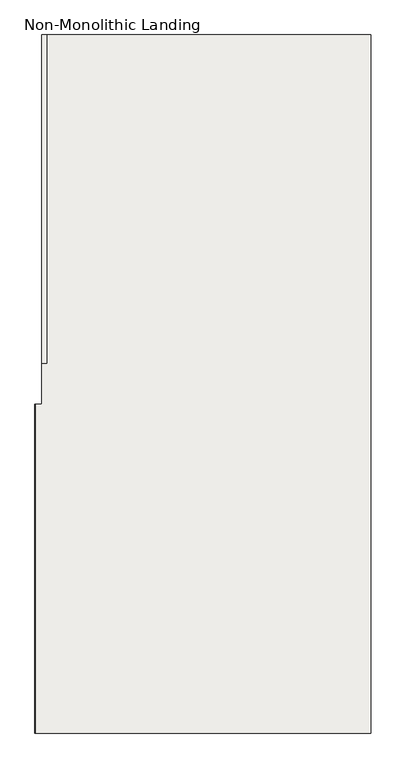
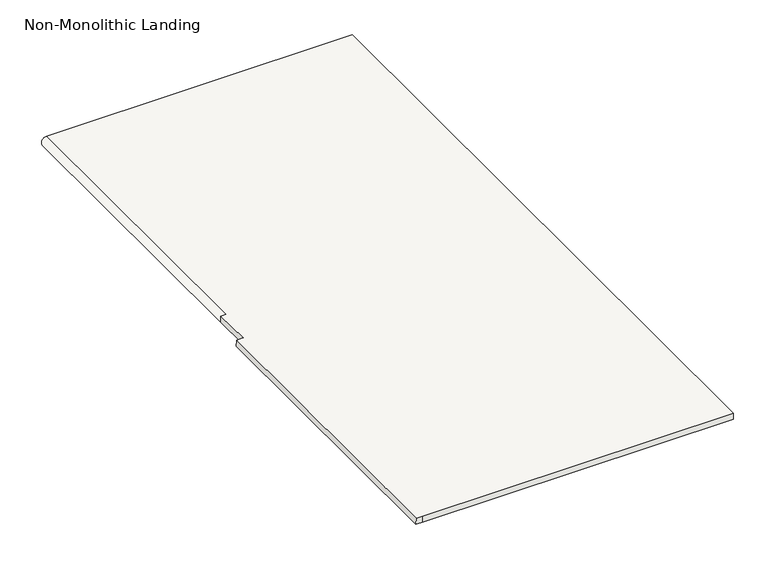
"""IFC4 building model written with IfcOpenShell, lengths in millimetres: slab geometry, Non-Monolithic Landing."""

from ifc_helpers import new_model, si_unit, frame, origin, place, context, project, spatial, circle_curve, source, transform, mapped, element, save
from ifc_brep_helpers import plane_surface, cylinder_surface, advanced_brep


def non_monolithic_landing_c74da7f8(model_context):
    return source(origin(), model_context, "Body", "AdvancedBrep", [
        advanced_brep(
        [(9872.4583908, 2257.2640673, 1676.4), (9871.3284975, 2257.2640673, 1651.0), (9871.3284975, 1038.0640673, 1651.0), (9872.4583908, 1038.0640673, 1676.4), (9917.4583908, 2407.2640673, 1676.4), (9897.4583908, 2407.2640673, 1676.4), (9897.4583908, 2257.2640673, 1676.4), (9897.4583908, 1038.0640673, 1676.4), (11116.6583908, 1038.0640673, 1676.4), (11116.6583908, 3626.4640673, 1676.4), (9917.4583908, 3626.4640673, 1676.4), (9897.4583908, 2257.2640673, 1651.0), (9897.4583908, 2407.2640673, 1651.0), (9898.2011843, 2407.2640673, 1651.0), (9917.4583908, 2407.2640673, 1651.0), (9917.4583908, 3626.4640673, 1651.0), (11116.6583908, 3626.4640673, 1651.0), (11116.6583908, 1038.0640673, 1651.0), (9897.4583908, 1038.0640673, 1651.0), (9897.4583908, 2407.2640673, 1656.4), (9917.4583908, 3626.4640673, 1636.4), (9917.4583908, 2407.2640673, 1636.4)],
        [
            (0, 1),
            (1, 2),
            (2, 3),
            (3, 0),
            (4, 5),
            (5, 6),
            (6, 0),
            (3, 7),
            (7, 8),
            (8, 9),
            (9, 10),
            (10, 4),
            (11, 12),
            (12, 13),
            (13, 14),
            (14, 15),
            (15, 16),
            (16, 17),
            (17, 18),
            (18, 2),
            (1, 11),
            (4, 19, circle_curve(frame((9917.4583908, 2407.2640673, 1656.4), z_axis=(0.0, -1.0, 0.0), x_axis=(1.0, 0.0, 0.0)), 20.0)),
            (19, 5),
            (12, 19),
            (19, 13, circle_curve(frame((9917.4583908, 2407.2640673, 1656.4), z_axis=(0.0, -1.0, 0.0), x_axis=(1.0, 0.0, 0.0)), 20.0)),
            (11, 6),
            (18, 7),
            (17, 8),
            (16, 9),
            (15, 20),
            (20, 10, circle_curve(frame((9917.4583908, 3626.4640673, 1656.4), z_axis=(0.0, 1.0, 0.0), x_axis=(1.0, 0.0, 0.0)), 20.0)),
            (21, 14),
            (13, 21, circle_curve(frame((9917.4583908, 2407.2640673, 1656.4), z_axis=(0.0, -1.0, 0.0), x_axis=(1.0, 0.0, 0.0)), 20.0)),
            (20, 21),
        ],
        [
            plane_surface(frame((9871.3284975, 2257.2640673, 1651.0), z_axis=(-0.9990120534936051, 0.0, 0.04444003796679731), x_axis=(0.0, -1.0, 0.0))),
            plane_surface(frame((9917.4583908, 3626.4640673, 1676.4), z_axis=(0.0, 0.0, 1.0), x_axis=(0.0, -1.0, 0.0))),
            plane_surface(frame((9917.4583908, 3626.4640673, 1651.0), z_axis=(0.0, 0.0, -1.0), x_axis=(0.0, 1.0, 0.0))),
            plane_surface(frame((9917.4583908, 2407.2640673, 1676.4), z_axis=(0.0, 1.0, 0.0), x_axis=(0.0, 0.0, -1.0))),
            plane_surface(frame((9897.4583908, 2407.2640673, 1676.4), z_axis=(-1.0, 0.0, 0.0), x_axis=(0.0, 0.0, -1.0))),
            plane_surface(frame((9897.4583908, 2257.2640673, 1676.4), z_axis=(0.0, 1.0, 0.0), x_axis=(0.0, 0.0, -1.0))),
            plane_surface(frame((9872.4583908, 1038.0640673, 1676.4), z_axis=(0.0, -1.0, 0.0), x_axis=(0.0, 0.0, -1.0))),
            plane_surface(frame((9897.4583908, 1038.0640673, 1676.4), z_axis=(0.0, -1.0, 0.0), x_axis=(0.0, 0.0, -1.0))),
            plane_surface(frame((11116.6583908, 1038.0640673, 1676.4), z_axis=(1.0, 0.0, 0.0), x_axis=(0.0, 0.0, -1.0))),
            plane_surface(frame((11116.6583908, 3626.4640673, 1676.4), z_axis=(0.0, 1.0, 0.0), x_axis=(0.0, 0.0, -1.0))),
            plane_surface(frame((9917.4583908, 2407.2640673, 1676.4), z_axis=(0.0, -1.0, 0.0), x_axis=(0.0, 0.0, 1.0))),
            cylinder_surface(frame((9917.4583908, 2407.2640673, 1656.4), z_axis=(0.0, -1.0, 0.0), x_axis=(1.0, 0.0, 0.0)), 20.0),
            plane_surface(frame((9917.4583908, 2407.2640673, 1636.4), z_axis=(1.0, 0.0, 0.0), x_axis=(0.0, 1.0, 0.0))),
        ],
        [
            (0, [[1, 2, 3, 4]]),
            (1, [[5, 6, 7, -4, 8, 9, 10, 11, 12]]),
            (2, [[13, 14, 15, 16, 17, 18, 19, 20, -2, 21]]),
            (3, [[-5, 22, 23]]),
            (3, [[-14, 24, 25]]),
            (4, [[-6, -23, -24, -13, 26]]),
            (5, [[-7, -26, -21, -1]]),
            (6, [[-8, -3, -20, 27]]),
            (7, [[-9, -27, -19, 28]]),
            (8, [[-10, -28, -18, 29]]),
            (9, [[-11, -29, -17, 30, 31]]),
            (10, [[32, -15, 33]]),
            (11, [[-31, 34, -33, -25, -22, -12]]),
            (12, [[-34, -30, -16, -32]]),
        ],
    ),
    ])


if __name__ == "__main__":
    model = new_model("IFC4")
    model_context = context("Model", 3, world=origin())
    ifc_project = project(units=[si_unit("LENGTHUNIT", "METRE", prefix="MILLI")], contexts=[model_context])
    site = spatial("IfcSite", under=ifc_project)
    building = spatial("IfcBuilding", under=site)
    placement = place(None, origin())
    non_monolithic_landing_shape = non_monolithic_landing_c74da7f8(model_context)
    element("IfcSlab", 1, ObjectType="Non-Monolithic Landing", at=placement, inside=building, context=model_context, shape_type="MappedRepresentation", body=[
        mapped(non_monolithic_landing_shape, transform((0.0, 0.0, 0.0), x_axis=(1.0, 0.0, 0.0), y_axis=(0.0, 1.0, 0.0), z_axis=(0.0, 0.0, 1.0))),
    ])
    save(model, "model.ifc")
